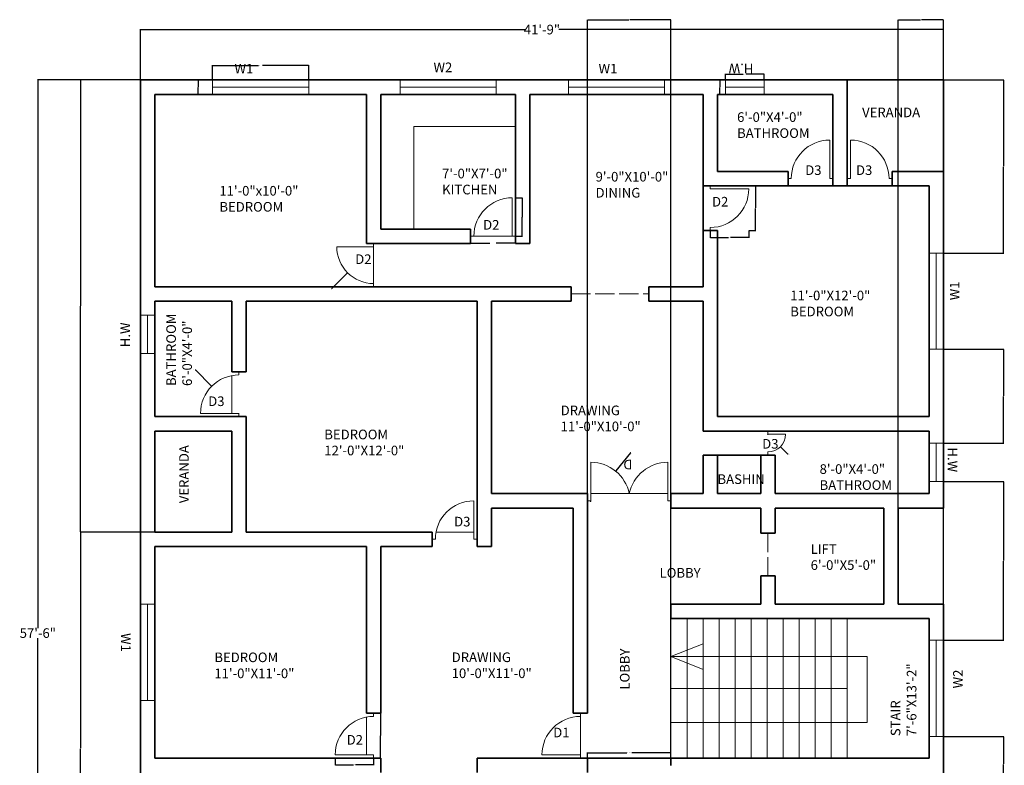
# Model space of a CAD drawing. Units: inches. Extents: x -51 to 563, y -718 to 47.
# Tile 2 of 2: x -51 to 563, y -418 to 47. Entities that reach past the tile are written whole.
import ezdxf

# ---------------------------------------------------------------- set-up
doc = ezdxf.new("R2010")
doc.units = ezdxf.units.IN
doc.header["$MEASUREMENT"] = 0
doc.linetypes.add('ACAD_ISO02W100', pattern=[15, 12, -3])
for name, color, linetype, lineweight in [('A-ANNO-DIMS', 2, 'Continuous', 18), ('A-ANNO-TEXT', 7, 'Continuous', 18), ('A-AREA-IDEN', 7, 'Continuous', 18), ('A-DOOR', 3, 'Continuous', 18), ('A-FLOR-CASE', 9, 'Continuous', 18), ('A-FLOR-STRS', 7, 'Continuous', 18), ('A-GLAZ', 164, 'Continuous', 18), ('A-WALL', 7, 'Continuous', 35), ('A-WALL-OPEN', 8, 'ACAD_ISO02W100', 13)]:
    doc.layers.add(name, color=color, linetype=linetype, lineweight=lineweight)
doc.styles.get("Standard").update_dxf_attribs({"font": 'arial.ttf'})
doc.dimstyles.get("Standard").update_dxf_attribs({"dimtxt": 0.18, "dimasz": 0.18, "dimexe": 0.18, "dimexo": 0.0625, "dimgap": 0.09, "dimtad": 0, "dimtih": 1, "dimtoh": 1, "dimdec": 0, "dimzin": 0, "dimdsep": 46, "dimlunit": 3, "dimtxsty": 'Standard', "dimcen": 0.09, "dimadec": 0, "dimazin": 0, "dimtfac": 1, "dimtdec": 0, "dimtofl": 0, "dimtmove": 0, "dimatfit": 3, "dimfxl": 1, "dimtolj": 1, "dimtzin": 0, "dimarcsym": 0})

# ---------------------------------------------------------------- blocks, each defined once
blk = doc.blocks.new('*D1')
at = {"layer": 'A-ANNO-DIMS', "color": 0, "lineweight": -2, "transparency": 16777216}
for p, q in [((24.24, 9.78), (24.24, 41.31)), ((24.42, 41.13), (264.22, 41.13)), ((525.06, 41.13), (285.25, 41.13)), ((525.24, 9.78), (525.24, 41.31))]:
    blk.add_line(p, q, dxfattribs=at)
at = {"layer": 'A-ANNO-DIMS', "color": 0, "transparency": 16777216}
for points in [[(24.42, 41.16), (24.42, 41.1), (24.24, 41.13)], [(525.06, 41.16), (525.06, 41.1), (525.24, 41.13)]]:
    blk.add_solid(points, dxfattribs=at)
at = {"layer": 'Defpoints', "color": 0, "transparency": 16777216}
for p in [(525.24, 41.13), (24.24, 9.71), (525.24, 9.71)]:
    blk.add_point(p, dxfattribs=at)
at = {"layer": 'A-ANNO-DIMS', "color": 0, "transparency": 16777216, "insert": (274.74, 41.13), "char_height": 6, "attachment_point": 5}
blk.add_mtext('\\A1;41\'-9"', dxfattribs=at)
blk = doc.blocks.new('*D2')
at = {"layer": 'A-ANNO-DIMS', "color": 0, "lineweight": -2, "transparency": 16777216}
for p, q in [((24.17, 9.71), (-39.93, 9.71)), ((-39.75, 9.53), (-39.75, -332.13)), ((-39.75, -680.11), (-39.75, -338.44)), ((24.17, -680.29), (-39.93, -680.29))]:
    blk.add_line(p, q, dxfattribs=at)
at = {"layer": 'A-ANNO-DIMS', "color": 0, "transparency": 16777216}
for points in [[(-39.78, 9.53), (-39.72, 9.53), (-39.75, 9.71)], [(-39.78, -680.11), (-39.72, -680.11), (-39.75, -680.29)]]:
    blk.add_solid(points, dxfattribs=at)
at = {"layer": 'Defpoints', "color": 0, "transparency": 16777216}
for p in [(24.24, 9.71), (-39.75, -680.29), (24.24, -680.29)]:
    blk.add_point(p, dxfattribs=at)
at = {"layer": 'A-ANNO-DIMS', "color": 0, "transparency": 16777216, "insert": (-39.75, -335.29), "char_height": 6, "attachment_point": 5}
blk.add_mtext('\\A1;57\'-6"', dxfattribs=at)
blk = doc.blocks.new('WIN-60IN')
for p, q in [((0, 9), (60, 9)), ((0, 0), (0, 9)), ((60, 9), (60, 0)), ((0, 4.5), (60, 4.5)), ((60, 0), (0, 0))]:
    blk.add_line(p, q)
blk = doc.blocks.new('WIN-24IN')
for p, q in [((0, 9), (24, 9)), ((0, 0), (0, 9)), ((24, 9), (24, 0)), ((0, 4.5), (24, 4.5)), ((24, 0), (0, 0))]:
    blk.add_line(p, q)
blk = doc.blocks.new('DOOR-24IN-CENTER-THRESHOLD')
for p, q in [((26, 0), (26, 24)), ((2, 0), (0, 0)), ((2, 0), (26, 0)), ((28, 0), (26, 0))]:
    blk.add_line(p, q)
blk.add_arc((26, 0), 24, 90, 180)
blk = doc.blocks.new('DOOR-24IN-SWING')
for p, q in [((26, 0), (26, 24)), ((2, 0), (0, 0)), ((28, 0), (26, 0))]:
    blk.add_line(p, q)
blk.add_arc((26, 0), 24, 90, 180)
blk = doc.blocks.new('DOOR-24IN-OFFSET-THRESHOLD')
for p, q in [((19.5, 25.57), (19.5, 2)), ((24, 26), (24, 28)), ((24, 2), (0, 2)), ((24, 0), (24, 2))]:
    blk.add_line(p, q)
blk.add_arc((24, 2), 24, 90, 180)
blk = doc.blocks.new('DOOR-48IN-PAIR')
for p, q in [((2, 0), (2, 24)), ((50, 0), (50, 24)), ((0, 0), (2, 0)), ((50, 0), (52, 0))]:
    blk.add_line(p, q)
for centre, start, end in [((2, -0.52), 11.81228, 90), ((50, -0.52), 90, 168.18772)]:
    blk.add_arc(centre, 24.52, start, end)
blk = doc.blocks.new('*D9')
at = {"layer": 'A-ANNO-DIMS', "color": 0, "lineweight": -2, "transparency": 16777216}
for p, q in [((69.24, 9.78), (69.24, 18.89)), ((69.42, 18.71), (98.01, 18.71)), ((129.06, 18.71), (100.47, 18.71)), ((129.24, 9.78), (129.24, 18.89))]:
    blk.add_line(p, q, dxfattribs=at)
at = {"layer": 'A-ANNO-DIMS', "color": 0, "transparency": 16777216}
for points in [[(69.42, 18.74), (69.42, 18.68), (69.24, 18.71)], [(129.06, 18.74), (129.06, 18.68), (129.24, 18.71)]]:
    blk.add_solid(points, dxfattribs=at)
at = {"layer": 'Defpoints', "color": 0, "transparency": 16777216}
for p in [(129.24, 18.71), (69.24, 9.71), (129.24, 9.71)]:
    blk.add_point(p, dxfattribs=at)
at = {"layer": 'A-ANNO-DIMS', "color": 0, "transparency": 16777216, "insert": (99.24, 18.71), "char_height": 0.18, "attachment_point": 5}
blk.add_mtext('\\A1;WINDOW 5\'-0" TYP.', dxfattribs=at)
blk = doc.blocks.new('*D10')
at = {"layer": 'A-ANNO-DIMS', "color": 0, "lineweight": -2, "transparency": 16777216}
for p, q in [((69.17, 9.71), (60.06, 9.71)), ((60.24, 9.53), (60.24, 5.4)), ((69.17, 0.71), (60.06, 0.71)), ((60.24, 0.89), (60.24, 5.03))]:
    blk.add_line(p, q, dxfattribs=at)
at = {"layer": 'A-ANNO-DIMS', "color": 0, "transparency": 16777216}
for points in [[(60.21, 9.53), (60.27, 9.53), (60.24, 9.71)], [(60.21, 0.89), (60.27, 0.89), (60.24, 0.71)]]:
    blk.add_solid(points, dxfattribs=at)
at = {"layer": 'Defpoints', "color": 0, "transparency": 16777216}
for p in [(60.24, 9.71), (69.24, 9.71), (69.24, 0.71)]:
    blk.add_point(p, dxfattribs=at)
at = {"layer": 'A-ANNO-DIMS', "color": 0, "transparency": 16777216, "insert": (60.24, 5.21), "char_height": 0.18, "attachment_point": 5}
blk.add_mtext('\\A1;0\'-9" TYP.', dxfattribs=at)
blk = doc.blocks.new('*D11')
at = {"layer": 'A-ANNO-DIMS', "color": 0, "lineweight": -2, "transparency": 16777216}
for p, q in [((389.26, 9.78), (389.26, 13.49)), ((389.44, 13.31), (400.31, 13.31)), ((413.08, 13.31), (402.21, 13.31)), ((413.26, 9.78), (413.26, 13.49))]:
    blk.add_line(p, q, dxfattribs=at)
at = {"layer": 'A-ANNO-DIMS', "color": 0, "transparency": 16777216}
for points in [[(389.44, 13.34), (389.44, 13.28), (389.26, 13.31)], [(413.08, 13.34), (413.08, 13.28), (413.26, 13.31)]]:
    blk.add_solid(points, dxfattribs=at)
at = {"layer": 'Defpoints', "color": 0, "transparency": 16777216}
for p in [(389.26, 13.31), (389.26, 9.71), (413.26, 9.71)]:
    blk.add_point(p, dxfattribs=at)
at = {"layer": 'A-ANNO-DIMS', "color": 0, "transparency": 16777216, "insert": (401.26, 13.31), "char_height": 0.18, "attachment_point": 5}
blk.add_mtext('\\A1;H.W. 2\'-0" TYP.', dxfattribs=at)
blk = doc.blocks.new('*D12')
at = {"layer": 'A-ANNO-DIMS', "color": 0, "lineweight": -2, "transparency": 16777216}
for p, q in [((389.2, 9.71), (385.48, 9.71)), ((385.66, 9.53), (385.66, 5.4)), ((389.2, 0.71), (385.48, 0.71)), ((385.66, 0.89), (385.66, 5.03))]:
    blk.add_line(p, q, dxfattribs=at)
at = {"layer": 'A-ANNO-DIMS', "color": 0, "transparency": 16777216}
for points in [[(385.63, 9.53), (385.69, 9.53), (385.66, 9.71)], [(385.63, 0.89), (385.69, 0.89), (385.66, 0.71)]]:
    blk.add_solid(points, dxfattribs=at)
at = {"layer": 'Defpoints', "color": 0, "transparency": 16777216}
for p in [(389.26, 9.71), (385.66, 0.71), (389.26, 0.71)]:
    blk.add_point(p, dxfattribs=at)
at = {"layer": 'A-ANNO-DIMS', "color": 0, "transparency": 16777216, "insert": (385.66, 5.21), "char_height": 0.18, "attachment_point": 5}
blk.add_mtext('\\A1;0\'-9" TYP.', dxfattribs=at)
blk = doc.blocks.new('*D13')
at = {"layer": 'A-ANNO-DIMS', "color": 0, "lineweight": -2, "transparency": 16777216}
for p, q in [((169.8, -385.29), (174.12, -385.29)), ((173.94, -385.47), (173.94, -399.1)), ((173.94, -413.11), (173.94, -399.47)), ((169.8, -413.29), (174.12, -413.29))]:
    blk.add_line(p, q, dxfattribs=at)
at = {"layer": 'A-ANNO-DIMS', "color": 0, "transparency": 16777216}
for points in [[(173.91, -385.47), (173.97, -385.47), (173.94, -385.29)], [(173.91, -413.11), (173.97, -413.11), (173.94, -413.29)]]:
    blk.add_solid(points, dxfattribs=at)
at = {"layer": 'Defpoints', "color": 0, "transparency": 16777216}
for p in [(169.74, -385.29), (173.94, -385.29), (169.74, -413.29)]:
    blk.add_point(p, dxfattribs=at)
at = {"layer": 'A-ANNO-DIMS', "color": 0, "transparency": 16777216, "insert": (173.94, -399.29), "char_height": 0.18, "attachment_point": 5}
blk.add_mtext('\\A1;OFFSET THRESHOLD 2\'-4" TYP.', dxfattribs=at)
blk = doc.blocks.new('*D14')
at = {"layer": 'A-ANNO-DIMS', "color": 0, "lineweight": -2, "transparency": 16777216}
for p, q in [((145.74, -413.35), (145.74, -417.67)), ((145.92, -417.49), (157.1, -417.49)), ((169.56, -417.49), (158.38, -417.49)), ((169.74, -413.35), (169.74, -417.67))]:
    blk.add_line(p, q, dxfattribs=at)
at = {"layer": 'A-ANNO-DIMS', "color": 0, "transparency": 16777216}
for points in [[(145.92, -417.46), (145.92, -417.52), (145.74, -417.49)], [(169.56, -417.46), (169.56, -417.52), (169.74, -417.49)]]:
    blk.add_solid(points, dxfattribs=at)
at = {"layer": 'Defpoints', "color": 0, "transparency": 16777216}
for p in [(145.74, -413.29), (169.74, -413.29), (169.74, -417.49)]:
    blk.add_point(p, dxfattribs=at)
at = {"layer": 'A-ANNO-DIMS', "color": 0, "transparency": 16777216, "insert": (157.74, -417.49), "char_height": 0.18, "attachment_point": 5}
blk.add_mtext('\\A1;2\'-0" TYP.', dxfattribs=at)
blk = doc.blocks.new('*D15')
at = {"layer": 'A-ANNO-DIMS', "color": 0, "lineweight": -2, "transparency": 16777216}
for p, q in [((403.8, -56.29), (408.12, -56.29)), ((407.94, -56.47), (407.94, -70.1)), ((407.94, -84.11), (407.94, -70.47)), ((403.8, -84.29), (408.12, -84.29))]:
    blk.add_line(p, q, dxfattribs=at)
at = {"layer": 'A-ANNO-DIMS', "color": 0, "transparency": 16777216}
for points in [[(407.91, -56.47), (407.97, -56.47), (407.94, -56.29)], [(407.91, -84.11), (407.97, -84.11), (407.94, -84.29)]]:
    blk.add_solid(points, dxfattribs=at)
at = {"layer": 'Defpoints', "color": 0, "transparency": 16777216}
for p in [(403.74, -56.29), (407.94, -56.29), (403.74, -84.29)]:
    blk.add_point(p, dxfattribs=at)
at = {"layer": 'A-ANNO-DIMS', "color": 0, "transparency": 16777216, "insert": (407.94, -70.29), "char_height": 0.18, "attachment_point": 5}
blk.add_mtext('\\A1;SWING DOOR 2\'-4" TYP.', dxfattribs=at)
blk = doc.blocks.new('*D16')
at = {"layer": 'A-ANNO-DIMS', "color": 0, "lineweight": -2, "transparency": 16777216}
for p, q in [((379.74, -84.35), (379.74, -88.67)), ((403.74, -84.35), (403.74, -88.67)), ((379.92, -88.49), (391.1, -88.49)), ((403.56, -88.49), (392.38, -88.49))]:
    blk.add_line(p, q, dxfattribs=at)
at = {"layer": 'A-ANNO-DIMS', "color": 0, "transparency": 16777216}
for points in [[(379.92, -88.46), (379.92, -88.52), (379.74, -88.49)], [(403.56, -88.46), (403.56, -88.52), (403.74, -88.49)]]:
    blk.add_solid(points, dxfattribs=at)
at = {"layer": 'Defpoints', "color": 0, "transparency": 16777216}
for p in [(379.74, -84.29), (403.74, -84.29), (403.74, -88.49)]:
    blk.add_point(p, dxfattribs=at)
at = {"layer": 'A-ANNO-DIMS', "color": 0, "transparency": 16777216, "insert": (391.74, -88.49), "char_height": 0.18, "attachment_point": 5}
blk.add_mtext('\\A1;2\'-0" TYP.', dxfattribs=at)
blk = doc.blocks.new('*D17')
at = {"layer": 'A-ANNO-DIMS', "color": 0, "lineweight": -2, "transparency": 16777216}
for p, q in [((230.24, -87.85), (230.24, -92.17)), ((230.42, -91.99), (242.24, -91.99)), ((258.06, -91.99), (246.24, -91.99)), ((258.24, -87.85), (258.24, -92.17))]:
    blk.add_line(p, q, dxfattribs=at)
at = {"layer": 'A-ANNO-DIMS', "color": 0, "transparency": 16777216}
for points in [[(230.42, -91.96), (230.42, -92.02), (230.24, -91.99)], [(258.06, -91.96), (258.06, -92.02), (258.24, -91.99)]]:
    blk.add_solid(points, dxfattribs=at)
at = {"layer": 'Defpoints', "color": 0, "transparency": 16777216}
for p in [(230.24, -87.79), (258.24, -87.79), (258.24, -91.99)]:
    blk.add_point(p, dxfattribs=at)
at = {"layer": 'A-ANNO-DIMS', "color": 0, "transparency": 16777216, "insert": (244.24, -91.99), "char_height": 0.18, "attachment_point": 5}
blk.add_mtext('\\A1;CENTER THRESHOLD 2\'-4" TYP.', dxfattribs=at)
blk = doc.blocks.new('*D18')
at = {"layer": 'A-ANNO-DIMS', "color": 0, "lineweight": -2, "transparency": 16777216}
for p, q in [((258.3, -63.79), (262.62, -63.79)), ((262.44, -63.97), (262.44, -75.6)), ((262.44, -87.61), (262.44, -75.97)), ((258.3, -87.79), (262.62, -87.79))]:
    blk.add_line(p, q, dxfattribs=at)
at = {"layer": 'A-ANNO-DIMS', "color": 0, "transparency": 16777216}
for points in [[(262.41, -63.97), (262.47, -63.97), (262.44, -63.79)], [(262.41, -87.61), (262.47, -87.61), (262.44, -87.79)]]:
    blk.add_solid(points, dxfattribs=at)
at = {"layer": 'Defpoints', "color": 0, "transparency": 16777216}
for p in [(258.24, -63.79), (262.44, -63.79), (258.24, -87.79)]:
    blk.add_point(p, dxfattribs=at)
at = {"layer": 'A-ANNO-DIMS', "color": 0, "transparency": 16777216, "insert": (262.44, -75.79), "char_height": 0.18, "attachment_point": 5}
blk.add_mtext('\\A1;2\'-0" TYP.', dxfattribs=at)
blk = doc.blocks.new('*D19')
at = {"layer": 'A-ANNO-DIMS', "color": 0, "lineweight": -2, "transparency": 16777216}
for p, q in [((303.24, -417.72), (303.24, -409.81)), ((303.42, -409.99), (327.69, -409.99)), ((355.06, -409.99), (330.79, -409.99)), ((355.24, -417.72), (355.24, -409.81))]:
    blk.add_line(p, q, dxfattribs=at)
at = {"layer": 'A-ANNO-DIMS', "color": 0, "transparency": 16777216}
for points in [[(303.42, -409.96), (303.42, -410.02), (303.24, -409.99)], [(355.06, -409.96), (355.06, -410.02), (355.24, -409.99)]]:
    blk.add_solid(points, dxfattribs=at)
at = {"layer": 'Defpoints', "color": 0, "transparency": 16777216}
for p in [(303.24, -409.99), (303.24, -417.79), (355.24, -417.79)]:
    blk.add_point(p, dxfattribs=at)
at = {"layer": 'A-ANNO-DIMS', "color": 0, "transparency": 16777216, "insert": (329.24, -409.99), "char_height": 0.18, "attachment_point": 5}
blk.add_mtext('\\A1;PAIRED DOOR 4\'-4" TYP.', dxfattribs=at)
blk = doc.blocks.new('*D25')
at = {"layer": 'A-ANNO-DIMS', "color": 0, "lineweight": -2, "transparency": 16777216}
for p, q in [((24.17, 9.71), (-13.34, 9.71)), ((-13.16, 9.53), (-13.16, -131.1)), ((-13.16, -272.11), (-13.16, -131.47)), ((33.17, -272.29), (-13.34, -272.29))]:
    blk.add_line(p, q, dxfattribs=at)
at = {"layer": 'A-ANNO-DIMS', "color": 0, "transparency": 16777216}
for points in [[(-13.19, 9.53), (-13.13, 9.53), (-13.16, 9.71)], [(-13.19, -272.11), (-13.13, -272.11), (-13.16, -272.29)]]:
    blk.add_solid(points, dxfattribs=at)
at = {"layer": 'Defpoints', "color": 0, "transparency": 16777216}
for p in [(24.24, 9.71), (-13.16, -272.29), (33.24, -272.29)]:
    blk.add_point(p, dxfattribs=at)
at = {"layer": 'A-ANNO-DIMS', "color": 0, "transparency": 16777216, "insert": (-13.16, -131.29), "char_height": 0.18, "attachment_point": 5}
blk.add_mtext('\\A1;23\'-6"', dxfattribs=at)
blk = doc.blocks.new('*D26')
at = {"layer": 'A-ANNO-DIMS', "color": 0, "lineweight": -2, "transparency": 16777216}
for p, q in [((33.17, -272.29), (-13.34, -272.29)), ((-13.16, -272.47), (-13.16, -407.1)), ((-13.16, -542.11), (-13.16, -407.47)), ((33.17, -542.29), (-13.34, -542.29))]:
    blk.add_line(p, q, dxfattribs=at)
at = {"layer": 'A-ANNO-DIMS', "color": 0, "transparency": 16777216}
for points in [[(-13.19, -272.47), (-13.13, -272.47), (-13.16, -272.29)], [(-13.19, -542.11), (-13.13, -542.11), (-13.16, -542.29)]]:
    blk.add_solid(points, dxfattribs=at)
at = {"layer": 'Defpoints', "color": 0, "transparency": 16777216}
for p in [(33.24, -272.29), (-13.16, -542.29), (33.24, -542.29)]:
    blk.add_point(p, dxfattribs=at)
at = {"layer": 'A-ANNO-DIMS', "color": 0, "transparency": 16777216, "insert": (-13.16, -407.29), "char_height": 0.18, "attachment_point": 5}
blk.add_mtext('\\A1;22\'-6"', dxfattribs=at)
blk = doc.blocks.new('*D28')
at = {"layer": 'A-ANNO-DIMS', "color": 0, "lineweight": -2, "transparency": 16777216}
for p, q in [((525.3, 9.71), (562.82, 9.71)), ((562.64, 9.53), (562.64, -44.1)), ((562.64, -98.11), (562.64, -44.47)), ((525.3, -98.29), (562.82, -98.29))]:
    blk.add_line(p, q, dxfattribs=at)
at = {"layer": 'A-ANNO-DIMS', "color": 0, "transparency": 16777216}
for points in [[(562.61, 9.53), (562.67, 9.53), (562.64, 9.71)], [(562.61, -98.11), (562.67, -98.11), (562.64, -98.29)]]:
    blk.add_solid(points, dxfattribs=at)
at = {"layer": 'Defpoints', "color": 0, "transparency": 16777216}
for p in [(525.24, 9.71), (525.24, -98.29), (562.64, -98.29)]:
    blk.add_point(p, dxfattribs=at)
at = {"layer": 'A-ANNO-DIMS', "color": 0, "transparency": 16777216, "insert": (562.64, -44.29), "char_height": 0.18, "attachment_point": 5}
blk.add_mtext('\\A1;9\'-0"', dxfattribs=at)
blk = doc.blocks.new('*D29')
at = {"layer": 'A-ANNO-DIMS', "color": 0, "lineweight": -2, "transparency": 16777216}
for p, q in [((525.3, -158.29), (562.82, -158.29)), ((562.64, -158.47), (562.64, -187.35)), ((562.64, -216.61), (562.64, -187.72)), ((525.3, -216.79), (562.82, -216.79))]:
    blk.add_line(p, q, dxfattribs=at)
at = {"layer": 'A-ANNO-DIMS', "color": 0, "transparency": 16777216}
for points in [[(562.61, -158.47), (562.67, -158.47), (562.64, -158.29)], [(562.61, -216.61), (562.67, -216.61), (562.64, -216.79)]]:
    blk.add_solid(points, dxfattribs=at)
at = {"layer": 'Defpoints', "color": 0, "transparency": 16777216}
for p in [(525.24, -158.29), (525.24, -216.79), (562.64, -216.79)]:
    blk.add_point(p, dxfattribs=at)
at = {"layer": 'A-ANNO-DIMS', "color": 0, "transparency": 16777216, "insert": (562.64, -187.54), "char_height": 0.18, "attachment_point": 5}
blk.add_mtext('\\A1;4\'-10 1/2"', dxfattribs=at)
blk = doc.blocks.new('*D30')
at = {"layer": 'A-ANNO-DIMS', "color": 0, "lineweight": -2, "transparency": 16777216}
for p, q in [((525.3, -240.79), (562.82, -240.79)), ((562.64, -240.97), (562.64, -290.1)), ((562.64, -339.61), (562.64, -290.47)), ((525.3, -339.79), (562.82, -339.79))]:
    blk.add_line(p, q, dxfattribs=at)
at = {"layer": 'A-ANNO-DIMS', "color": 0, "transparency": 16777216}
for points in [[(562.61, -240.97), (562.67, -240.97), (562.64, -240.79)], [(562.61, -339.61), (562.67, -339.61), (562.64, -339.79)]]:
    blk.add_solid(points, dxfattribs=at)
at = {"layer": 'Defpoints', "color": 0, "transparency": 16777216}
for p in [(525.24, -240.79), (525.24, -339.79), (562.64, -339.79)]:
    blk.add_point(p, dxfattribs=at)
at = {"layer": 'A-ANNO-DIMS', "color": 0, "transparency": 16777216, "insert": (562.64, -290.29), "char_height": 0.18, "attachment_point": 5}
blk.add_mtext('\\A1;8\'-3"', dxfattribs=at)
blk = doc.blocks.new('*D31')
at = {"layer": 'A-ANNO-DIMS', "color": 0, "lineweight": -2, "transparency": 16777216}
for p, q in [((525.3, -399.79), (562.82, -399.79)), ((562.64, -399.97), (562.64, -416.85)), ((562.64, -434.11), (562.64, -417.22)), ((525.3, -434.29), (562.82, -434.29))]:
    blk.add_line(p, q, dxfattribs=at)
at = {"layer": 'A-ANNO-DIMS', "color": 0, "transparency": 16777216}
for points in [[(562.61, -399.97), (562.67, -399.97), (562.64, -399.79)], [(562.61, -434.11), (562.67, -434.11), (562.64, -434.29)]]:
    blk.add_solid(points, dxfattribs=at)
at = {"layer": 'Defpoints', "color": 0, "transparency": 16777216}
for p in [(525.24, -399.79), (525.24, -434.29), (562.64, -434.29)]:
    blk.add_point(p, dxfattribs=at)
at = {"layer": 'A-ANNO-DIMS', "color": 0, "transparency": 16777216, "insert": (562.64, -417.04), "char_height": 0.18, "attachment_point": 5}
blk.add_mtext('\\A1;2\'-10 1/2"', dxfattribs=at)
blk = doc.blocks.new('*D33')
at = {"layer": 'A-ANNO-DIMS', "color": 0, "lineweight": -2, "transparency": 16777216}
for p, q in [((497.04, -317.22), (497.04, 47.29)), ((497.22, 47.11), (510.81, 47.11)), ((525.06, 47.11), (511.47, 47.11)), ((525.24, -317.22), (525.24, 47.29))]:
    blk.add_line(p, q, dxfattribs=at)
at = {"layer": 'A-ANNO-DIMS', "color": 0, "transparency": 16777216}
for points in [[(497.22, 47.14), (497.22, 47.08), (497.04, 47.11)], [(525.06, 47.14), (525.06, 47.08), (525.24, 47.11)]]:
    blk.add_solid(points, dxfattribs=at)
at = {"layer": 'Defpoints', "color": 0, "transparency": 16777216}
for p in [(525.24, 47.11), (497.04, -317.29), (525.24, -317.29)]:
    blk.add_point(p, dxfattribs=at)
at = {"layer": 'A-ANNO-DIMS', "color": 0, "transparency": 16777216, "insert": (511.14, 47.11), "char_height": 0.18, "attachment_point": 5}
blk.add_mtext('\\A1;2\'-4"', dxfattribs=at)
blk = doc.blocks.new('*D34')
at = {"layer": 'A-ANNO-DIMS', "color": 0, "lineweight": -2, "transparency": 16777216}
for p, q in [((303.24, -385.22), (303.24, 47.29)), ((303.42, 47.11), (328.9, 47.11)), ((355.06, 47.11), (329.57, 47.11)), ((355.24, -413.22), (355.24, 47.29))]:
    blk.add_line(p, q, dxfattribs=at)
at = {"layer": 'A-ANNO-DIMS', "color": 0, "transparency": 16777216}
for points in [[(303.42, 47.14), (303.42, 47.08), (303.24, 47.11)], [(355.06, 47.14), (355.06, 47.08), (355.24, 47.11)]]:
    blk.add_solid(points, dxfattribs=at)
at = {"layer": 'Defpoints', "color": 0, "transparency": 16777216}
for p in [(355.24, 47.11), (303.24, -385.29), (355.24, -413.29)]:
    blk.add_point(p, dxfattribs=at)
at = {"layer": 'A-ANNO-DIMS', "color": 0, "transparency": 16777216, "insert": (329.24, 47.11), "char_height": 0.18, "attachment_point": 5}
blk.add_mtext('\\A1;4\'-4"', dxfattribs=at)
blk = doc.blocks.new('*D35')
at = {"layer": 'A-ANNO-DIMS', "color": 0, "lineweight": -2, "transparency": 16777216}
for p, q in [((329.97, -222.86), (320.81, -234.14)), ((330.15, -222.86), (329.97, -222.86)), ((305.15, -253.31), (305.33, -253.31)), ((305.24, -253.4), (305.24, -253.22))]:
    blk.add_line(p, q, dxfattribs=at)
at = {"layer": 'A-ANNO-DIMS', "color": 0, "transparency": 16777216}
blk.add_solid([(320.79, -234.12), (320.83, -234.15), (320.7, -234.28)], dxfattribs=at)
at = {"layer": 'Defpoints', "color": 0, "transparency": 16777216}
for p in [(320.7, -234.28), (305.24, -253.31)]:
    blk.add_point(p, dxfattribs=at)
at = {"layer": 'A-ANNO-DIMS', "color": 0, "transparency": 16777216, "insert": (330.98, -222.86), "char_height": 0.18, "attachment_point": 5}
blk.add_mtext('\\A1;4X R2\'-0 1/2"', dxfattribs=at)
blk = doc.blocks.new('*D36')
at = {"layer": 'A-ANNO-DIMS', "color": 0, "lineweight": -2, "transparency": 16777216}
for p, q in [((58.4, -171.13), (58.58, -171.13)), ((58.58, -171.13), (68.64, -181.19)), ((85.65, -198.29), (85.83, -198.29)), ((85.74, -198.38), (85.74, -198.2))]:
    blk.add_line(p, q, dxfattribs=at)
at = {"layer": 'A-ANNO-DIMS', "color": 0, "transparency": 16777216}
blk.add_solid([(68.66, -181.17), (68.62, -181.21), (68.77, -181.32)], dxfattribs=at)
at = {"layer": 'Defpoints', "color": 0, "transparency": 16777216}
for p in [(68.77, -181.32), (85.74, -198.29)]:
    blk.add_point(p, dxfattribs=at)
at = {"layer": 'A-ANNO-DIMS', "color": 0, "transparency": 16777216, "insert": (57.8, -171.13), "char_height": 0.18, "attachment_point": 5}
blk.add_mtext('\\A1;7X R2\'-0"', dxfattribs=at)
blk = doc.blocks.new('*D38')
at = {"layer": 'A-ANNO-DIMS', "color": 0, "lineweight": -2, "transparency": 16777216}
for p, q in [((169.65, -94.29), (169.83, -94.29)), ((169.74, -94.38), (169.74, -94.2)), ((143.71, -120.31), (153.35, -110.68)), ((143.53, -120.31), (143.71, -120.31))]:
    blk.add_line(p, q, dxfattribs=at)
at = {"layer": 'A-ANNO-DIMS', "color": 0, "transparency": 16777216}
blk.add_solid([(153.32, -110.66), (153.37, -110.7), (153.47, -110.55)], dxfattribs=at)
at = {"layer": 'Defpoints', "color": 0, "transparency": 16777216}
for p in [(169.74, -94.29), (153.47, -110.55)]:
    blk.add_point(p, dxfattribs=at)
at = {"layer": 'A-ANNO-DIMS', "color": 0, "transparency": 16777216, "insert": (143.05, -120.31), "char_height": 0.18, "attachment_point": 5}
blk.add_mtext('\\A1;R1\'-11"', dxfattribs=at)
blk = doc.blocks.new('*D40')
at = {"layer": 'A-ANNO-DIMS', "color": 0, "lineweight": -2, "transparency": 16777216}
for p, q in [((415.65, -211.29), (415.83, -211.29)), ((415.74, -211.38), (415.74, -211.2)), ((428.18, -223.73), (423.64, -219.19)), ((428.36, -223.73), (428.18, -223.73))]:
    blk.add_line(p, q, dxfattribs=at)
at = {"layer": 'A-ANNO-DIMS', "color": 0, "transparency": 16777216}
blk.add_solid([(423.66, -219.17), (423.62, -219.21), (423.51, -219.06)], dxfattribs=at)
at = {"layer": 'Defpoints', "color": 0, "transparency": 16777216}
for p in [(415.74, -211.29), (423.51, -219.06)]:
    blk.add_point(p, dxfattribs=at)
at = {"layer": 'A-ANNO-DIMS', "color": 0, "transparency": 16777216, "insert": (428.85, -223.73), "char_height": 0.18, "attachment_point": 5}
blk.add_mtext('\\A1;R0\'-11"', dxfattribs=at)

msp = doc.modelspace()

# ---------------------------------------------------------------- linework, layer by layer
at = {"layer": 'A-DOOR'}
for p, q in [((169.74, -94.29), (146.74, -94.29)), ((169.74, -92.29), (169.74, -94.29)), ((169.74, -94.29), (169.74, -117.29)), ((169.74, -119.29), (169.74, -117.29)), ((415.74, -209.29), (415.74, -211.29)), ((415.74, -211.29), (426.74, -211.29)), ((415.74, -224.29), (415.74, -222.29)), ((305.24, -248.29), (353.24, -248.29))]:
    msp.add_line(p, q, dxfattribs=at)
for centre, radius, start, end in [((169.74, -94.29), 23, 180, 270), ((415.74, -211.29), 11, 270, 0)]:
    msp.add_arc(centre, radius, start, end, dxfattribs=at)
at = {"layer": 'A-FLOR-CASE'}
for p, q in [((258.24, -19.3), (194.72, -19.3)), ((194.72, -19.3), (194.72, -83.29))]:
    msp.add_line(p, q, dxfattribs=at)
at = {"layer": 'A-FLOR-STRS'}
for p, q in [((355.24, -326.29), (355.24, -413.29)), ((365.24, -326.29), (365.24, -413.29)), ((375.24, -326.29), (375.24, -413.29)), ((385.24, -326.29), (385.24, -413.29)), ((395.24, -326.29), (395.24, -413.29)), ((405.24, -326.29), (405.24, -413.29)), ((415.24, -326.29), (415.24, -413.29)), ((425.24, -326.29), (425.24, -413.29)), ((435.24, -326.29), (435.24, -413.29)), ((445.24, -326.29), (445.24, -413.29)), ((455.24, -326.29), (455.24, -413.29)), ((465.24, -326.29), (465.24, -413.29)), ((355.24, -349.99), (375.24, -341.96)), ((477.63, -349.99), (355.24, -349.99)), ((355.24, -349.99), (375.24, -358.03)), ((477.63, -391.11), (477.63, -349.99)), ((465.24, -369.79), (355.24, -369.79)), ((355.24, -391.11), (477.63, -391.11))]:
    msp.add_line(p, q, dxfattribs=at)
at = {"layer": 'A-WALL'}
for p, q in [((24.24, 9.71), (24.24, -680.29)), ((24.24, 9.71), (525.24, 9.71)), ((465.24, 9.71), (465.24, -47.29)), ((525.24, 9.71), (525.24, -119.29)), ((33.24, 0.71), (165.24, 0.71)), ((33.24, 0.71), (33.24, -119.29)), ((165.24, 0.71), (165.24, -92.29)), ((174.24, 0.71), (174.24, -83.29)), ((174.24, 0.71), (258.24, 0.71)), ((258.24, 0.71), (258.24, -83.29)), ((267.24, 0.71), (267.24, -92.29)), ((267.24, 0.71), (375.24, 0.71)), ((375.24, 0.71), (375.24, -119.29)), ((384.24, 0.71), (384.24, -47.29)), ((384.24, 0.71), (456.24, 0.71)), ((456.24, 0.71), (456.24, -47.29)), ((384.24, -47.29), (428.24, -47.29)), ((428.24, -51.79), (428.24, -47.29)), ((456.24, -47.29), (456.24, -56.29)), ((465.24, -47.29), (465.24, -56.29)), ((493.24, -47.29), (525.24, -47.29)), ((493.24, -51.79), (493.24, -47.29)), ((428.24, -51.79), (428.24, -56.29)), ((493.24, -51.79), (493.24, -56.29)), ((384.24, -56.29), (375.24, -56.29)), ((384.24, -56.29), (516.24, -56.29)), ((516.24, -56.29), (516.24, -119.29)), ((516.24, -56.29), (516.24, -200.29)), ((525.24, -56.29), (525.24, -257.29)), ((174.24, -83.29), (230.24, -83.29)), ((230.24, -87.79), (230.24, -83.29)), ((258.24, -83.29), (258.24, -92.29)), ((379.74, -84.29), (375.24, -84.29)), ((379.74, -84.29), (384.24, -84.29)), ((384.24, -84.29), (384.24, -128.29)), ((230.24, -87.79), (230.24, -92.29)), ((165.24, -92.29), (230.24, -92.29)), ((258.24, -92.29), (267.24, -92.29)), ((33.24, -119.29), (292.92, -119.29)), ((292.92, -119.29), (292.92, -128.29)), ((341.33, -119.29), (341.33, -128.29)), ((341.33, -119.29), (375.24, -119.29)), ((33.24, -128.29), (81.24, -128.29)), ((33.24, -128.29), (33.24, -200.29)), ((81.24, -128.29), (81.24, -172.29)), ((90.24, -128.29), (90.24, -172.29)), ((90.24, -128.29), (234.24, -128.29)), ((234.24, -128.29), (234.24, -272.29)), ((243.24, -128.29), (243.24, -248.29)), ((243.24, -128.29), (292.92, -128.29)), ((341.33, -128.29), (375.24, -128.29)), ((375.24, -128.29), (375.24, -209.29)), ((384.24, -128.29), (384.24, -200.29)), ((85.74, -172.29), (81.24, -172.29)), ((85.74, -172.29), (90.24, -172.29)), ((33.24, -200.29), (81.24, -200.29)), ((81.24, -200.29), (90.24, -200.29)), ((90.24, -200.29), (90.24, -272.29)), ((384.24, -200.29), (516.24, -200.29)), ((33.24, -209.29), (81.24, -209.29)), ((33.24, -209.29), (33.24, -272.29)), ((81.24, -209.29), (81.24, -272.29)), ((375.24, -209.29), (516.24, -209.29)), ((516.24, -209.29), (516.24, -248.29)), ((420.24, -224.29), (375.24, -224.29)), ((375.24, -224.29), (375.24, -248.29)), ((384.24, -224.29), (384.24, -248.29)), ((411.24, -224.29), (411.24, -248.29)), ((420.24, -224.29), (420.24, -248.29)), ((243.24, -248.29), (303.24, -248.29)), ((303.24, -257.29), (303.24, -248.29)), ((355.24, -252.79), (355.24, -248.29)), ((355.24, -248.29), (375.24, -248.29)), ((384.24, -248.29), (411.24, -248.29)), ((420.24, -248.29), (516.24, -248.29)), ((243.24, -257.29), (294.24, -257.29)), ((243.24, -257.29), (243.24, -281.29)), ((294.24, -257.29), (294.24, -385.29)), ((303.24, -257.29), (303.24, -385.29)), ((355.24, -252.79), (355.24, -257.29)), ((355.24, -257.29), (411.24, -257.29)), ((411.24, -257.29), (411.24, -272.91)), ((420.24, -257.29), (420.24, -272.91)), ((420.24, -257.29), (488.04, -257.29)), ((488.04, -257.29), (488.04, -317.29)), ((497.04, -257.29), (497.04, -317.29)), ((497.04, -257.29), (525.24, -257.29)), ((33.24, -272.29), (81.24, -272.29)), ((90.24, -272.29), (206.24, -272.29)), ((206.24, -276.79), (206.24, -272.29)), ((234.24, -272.29), (234.24, -281.29)), ((420.24, -272.91), (411.24, -272.91)), ((33.24, -281.29), (165.24, -281.29)), ((33.24, -281.29), (33.24, -413.29)), ((165.24, -281.29), (165.24, -385.29)), ((174.24, -281.29), (174.24, -385.29)), ((174.24, -281.29), (206.24, -281.29)), ((206.24, -276.79), (206.24, -281.29)), ((234.24, -281.29), (243.24, -281.29)), ((411.24, -299.54), (420.24, -299.54)), ((411.24, -299.54), (411.24, -317.29)), ((420.24, -299.54), (420.24, -317.29)), ((355.24, -317.29), (411.24, -317.29)), ((355.24, -317.29), (355.24, -326.29)), ((420.24, -317.29), (488.04, -317.29)), ((497.04, -317.29), (525.24, -317.29)), ((525.24, -317.29), (525.24, -680.29)), ((355.24, -326.29), (516.24, -326.29)), ((516.24, -326.29), (516.24, -413.29)), ((169.74, -385.29), (165.24, -385.29)), ((169.74, -385.29), (174.24, -385.29)), ((298.74, -385.29), (294.24, -385.29)), ((298.74, -385.29), (303.24, -385.29)), ((33.24, -413.29), (165.24, -413.29)), ((165.24, -413.29), (174.24, -413.29)), ((174.24, -413.29), (174.24, -422.29)), ((234.24, -413.29), (294.24, -413.29)), ((234.24, -422.29), (234.24, -413.29)), ((294.24, -413.29), (303.24, -413.29)), ((303.24, -413.29), (516.24, -413.29)), ((303.24, -413.29), (303.24, -422.29)), ((355.24, -417.79), (355.24, -413.29))]:
    msp.add_line(p, q, dxfattribs=at)
at = {"layer": 'A-WALL-OPEN'}
for p, q in [((292.92, -123.79), (341.33, -123.79)), ((415.74, -272.91), (415.74, -299.54))]:
    msp.add_line(p, q, dxfattribs=at)

# ---------------------------------------------------------------- block references
at = {"layer": 'A-DOOR'}
for name, p in [('DOOR-24IN-SWING', (428.24, -51.79)), ('DOOR-24IN-CENTER-THRESHOLD', (230.24, -87.79)), ('DOOR-24IN-OFFSET-THRESHOLD', (61.74, -200.29)), ('DOOR-48IN-PAIR', (303.24, -252.79)), ('DOOR-24IN-OFFSET-THRESHOLD', (145.74, -413.29))]:
    msp.add_blockref(name, p, dxfattribs=at)
at = {"layer": 'A-DOOR', "extrusion": (0, 0, -1), "zscale": -1}
msp.add_blockref('DOOR-24IN-SWING', (-493.24, -51.79), dxfattribs=at)
for name, p, rotation in [('DOOR-24IN-SWING', (-379.74, -84.29), 90.00000000000006), ('DOOR-24IN-OFFSET-THRESHOLD', (-234.24, -252.79), 269.9999999999998), ('DOOR-24IN-CENTER-THRESHOLD', (-298.74, -385.29), 270)]:
    msp.add_blockref(name, p, dxfattribs=dict(at, rotation=rotation))
at = {"layer": 'A-GLAZ'}
for p in [(69.24, 0.71), (186.24, 0.71), (291.24, 0.71)]:
    msp.add_blockref('WIN-60IN', p, dxfattribs=at)
for name, p, rotation in [('WIN-24IN', (413.26, 9.71), 180), ('WIN-60IN', (525.24, -158.29), 90.00000000000003), ('WIN-24IN', (24.24, -137), 269.9999999999995), ('WIN-24IN', (516.24, -216.79), 269.9999999999996), ('WIN-60IN', (33.24, -377.29), 89.99999999999996), ('WIN-60IN', (525.24, -399.79), 89.99999999999996)]:
    msp.add_blockref(name, p, dxfattribs=dict(at, rotation=rotation))

# ---------------------------------------------------------------- texts
at = {"layer": 'A-ANNO-TEXT', "char_height": 6, "attachment_point": 1}
for s, insert in [('W1', (82.94, 19.76)), ('W2', (207.08, 20.56)), ('W1', (310.05, 19.76)), ('D3', (438.97, -43.55)), ('D3', (470.65, -43.55)), ('D2', (380.82, -63.23)), ('D2', (238.06, -77.65)), ('D2', (158.24, -99.08)), ('D3', (66.55, -187.68)), ('D3', (412.12, -214.24)), ('D3', (219.96, -262.77)), ('D2', (152.92, -398.87)), ('D1', (281.77, -394.32))]:
    msp.add_mtext(s, dxfattribs=dict(at, insert=insert))
for s, insert, rotation in [('H.W', (406.64, 13.84), 180), ('W1', (529.19, -127.7), 90), ('H.W', (11.8, -156.98), 90), ('H.W', (533.93, -219.52), 270), ('D', (331.15, -233.2), 180), ('W1', (18.21, -335.29), 270), ('W2', (531.26, -369.79), 90)]:
    msp.add_mtext(s, dxfattribs=dict(at, insert=insert, rotation=rotation))
at = {"layer": 'A-AREA-IDEN', "char_height": 6, "attachment_point": 1}
for s, insert in [('6\'-0"X4\'-0"\\PBATHROOM', (396.47, -10.45)), ('VERANDA', (474.45, -7.54)), ('7\'-0"X7\'-0"\\PKITCHEN', (212.43, -45.66)), ('11\'-0"x10\'-0"\\PBEDROOM', (73.51, -56.42)), ('11\'-0"X12\'-0"\\PBEDROOM', (429.64, -121.72)), ('DRAWING\\P11\'-0"X10\'-0"', (286.41, -193.39)), ('BEDROOM\\P12\'-0"X12\'-0"', (138.96, -208.41)), ('8\'-0"X4\'-0"\\PBATHROOM', (447.94, -229.99)), ('BASHIN', (384.24, -236.29)), ('LIFT\\P6\'-0"X5\'-0"', (442.35, -279.87)), ('LOBBY', (348.12, -294.71)), ('BEDROOM\\P11\'-0"X11\'-0"', (70.38, -347.42)), ('DRAWING\\P10\'-0"X11\'-0"', (218.43, -347.37))]:
    msp.add_mtext(s, dxfattribs=dict(at, insert=insert))
at = {"layer": 'A-AREA-IDEN', "insert": (308.19, -47.65), "char_height": 6, "width": 1.4297, "attachment_point": 1}
msp.add_mtext('9\'-0"X10\'-0"\\PDINING', dxfattribs=at)
at = {"layer": 'A-AREA-IDEN', "char_height": 6, "attachment_point": 1, "rotation": 90}
for s, insert in [('BATHROOM\\P6\'-0"X4\'-0"', (40.4, -181.19)), ('VERANDA', (48.43, -254.3)), ('STAIR\\P7\'-6"X13\'-2"', (492.34, -399.6))]:
    msp.add_mtext(s, dxfattribs=dict(at, insert=insert))
at = {"layer": 'A-AREA-IDEN', "insert": (323.39, -370.58), "char_height": 6, "attachment_point": 1, "rotation": 90}
msp.add_mtext_dynamic_manual_height_columns('LOBBY', width=2.2613, gutter_width=1, heights=[0], dxfattribs=at)

# ---------------------------------------------------------------- dimensions: what is measured, and where the dimension line sits
at = {"layer": 'A-ANNO-DIMS'}
for base, p1, p2, override, picture, middle in [((525.24, 41.13), (24.24, 9.71), (525.24, 9.71), {"dimtxt": 6, "dimclrd": 0, "dimclre": 0, "dimclrt": 0}, '*D1', (274.74, 41.13)), ((355.24, 47.11), (303.24, -385.29), (355.24, -413.29), {"dimdec": 1, "dimlfac": 1, "dimrnd": 0, "dimzin": 1, "dimdsep": 46, "dimlunit": 4, "dimfrac": 2}, '*D34', (329.24, 47.11)), ((525.24, 47.11), (497.04, -317.29), (525.24, -317.29), {"dimdec": 1, "dimlfac": 1, "dimrnd": 0, "dimzin": 1, "dimdsep": 46, "dimlunit": 4, "dimfrac": 2}, '*D33', (511.14, 47.11))]:
    dim = msp.add_linear_dim(base=base, p1=p1, p2=p2, dimstyle='Standard', override=override, dxfattribs=at)
    dim.commit()
    dim.dimension.update_dxf_attribs({"geometry": picture, "text_midpoint": middle})
for base, p1, p2, text, picture, middle in [((129.24, 18.71), (69.24, 9.71), (129.24, 9.71), 'WINDOW <> TYP.', '*D9', (99.24, 18.71)), ((403.74, -88.49), (379.74, -84.29), (403.74, -84.29), '<> TYP.', '*D16', (391.74, -88.49)), ((258.24, -91.99), (230.24, -87.79), (258.24, -87.79), 'CENTER THRESHOLD <> TYP.', '*D17', (244.24, -91.99)), ((169.74, -417.49), (145.74, -413.29), (169.74, -413.29), '<> TYP.', '*D14', (157.74, -417.49))]:
    dim = msp.add_linear_dim(base=base, p1=p1, p2=p2, text=text, dimstyle='Standard', override={"dimdec": 1, "dimlfac": 1, "dimrnd": 0, "dimzin": 1, "dimdsep": 46, "dimlunit": 4, "dimfrac": 2}, dxfattribs=at)
    dim.commit()
    dim.dimension.update_dxf_attribs({"geometry": picture, "text_midpoint": middle})
for base, p1, p2, angle, text, picture, middle in [((389.26, 13.31), (413.26, 9.71), (389.26, 9.71), 180, 'H.W. <> TYP.', '*D11', (401.26, 13.31)), ((60.24, 9.71), (69.24, 0.71), (69.24, 9.71), 90, '<> TYP.', '*D10', (60.24, 5.21)), ((385.66, 0.71), (389.26, 9.71), (389.26, 0.71), 270, '<> TYP.', '*D12', (385.66, 5.21)), ((407.94, -56.29), (403.74, -84.29), (403.74, -56.29), 90, 'SWING DOOR <> TYP.', '*D15', (407.94, -70.29)), ((262.44, -63.79), (258.24, -87.79), (258.24, -63.79), 90, '<> TYP.', '*D18', (262.44, -75.79)), ((173.94, -385.29), (169.74, -413.29), (169.74, -385.29), 90, 'OFFSET THRESHOLD <> TYP.', '*D13', (173.94, -399.29)), ((303.24, -409.99), (355.24, -417.79), (303.24, -417.79), 180, 'PAIRED DOOR <> TYP.', '*D19', (329.24, -409.99))]:
    dim = msp.add_linear_dim(base=base, p1=p1, p2=p2, angle=angle, text=text, dimstyle='Standard', override={"dimdec": 1, "dimlfac": 1, "dimrnd": 0, "dimzin": 1, "dimdsep": 46, "dimlunit": 4, "dimfrac": 2}, dxfattribs=at)
    dim.commit()
    dim.dimension.update_dxf_attribs({"geometry": picture, "text_midpoint": middle})
for base, p1, p2, override, picture, middle in [((-39.75, -680.29), (24.24, 9.71), (24.24, -680.29), {"dimtxt": 6, "dimclrd": 0, "dimclre": 0, "dimclrt": 0}, '*D2', (-39.75, -335.29)), ((-13.16, -272.29), (24.24, 9.71), (33.24, -272.29), {"dimdec": 1, "dimlfac": 1, "dimrnd": 0, "dimzin": 1, "dimdsep": 46, "dimlunit": 4, "dimfrac": 2}, '*D25', (-13.16, -131.29)), ((562.64, -98.29), (525.24, 9.71), (525.24, -98.29), {"dimdec": 1, "dimlfac": 1, "dimrnd": 0, "dimzin": 1, "dimdsep": 46, "dimlunit": 4, "dimfrac": 2}, '*D28', (562.64, -44.29)), ((562.64, -216.79), (525.24, -158.29), (525.24, -216.79), {"dimdec": 1, "dimlfac": 1, "dimrnd": 0, "dimzin": 1, "dimdsep": 46, "dimlunit": 4, "dimfrac": 2}, '*D29', (562.64, -187.54)), ((562.64, -339.79), (525.24, -240.79), (525.24, -339.79), {"dimdec": 1, "dimlfac": 1, "dimrnd": 0, "dimzin": 1, "dimdsep": 46, "dimlunit": 4, "dimfrac": 2}, '*D30', (562.64, -290.29)), ((-13.16, -542.29), (33.24, -272.29), (33.24, -542.29), {"dimdec": 1, "dimlfac": 1, "dimrnd": 0, "dimzin": 1, "dimdsep": 46, "dimlunit": 4, "dimfrac": 2}, '*D26', (-13.16, -407.29)), ((562.64, -434.29), (525.24, -399.79), (525.24, -434.29), {"dimdec": 1, "dimlfac": 1, "dimrnd": 0, "dimzin": 1, "dimdsep": 46, "dimlunit": 4, "dimfrac": 2}, '*D31', (562.64, -417.04))]:
    dim = msp.add_linear_dim(base=base, p1=p1, p2=p2, angle=90, dimstyle='Standard', override=override, dxfattribs=at)
    dim.commit()
    dim.dimension.update_dxf_attribs({"geometry": picture, "text_midpoint": middle})
for center, mpoint, picture, middle in [((169.74, -94.29), (153.47, -110.55), '*D38', (143.05, -120.31)), ((415.74, -211.29), (423.51, -219.06), '*D40', (428.85, -223.73))]:
    dim = msp.add_radius_dim(center=center, mpoint=mpoint, dimstyle='Standard', override={"dimdec": 1, "dimlfac": 1, "dimrnd": 0, "dimzin": 1, "dimdsep": 46, "dimlunit": 4, "dimfrac": 2}, dxfattribs=at)
    dim.commit()
    dim.dimension.update_dxf_attribs({"geometry": picture, "text_midpoint": middle, "dimtype": 164})
for center, mpoint, text, picture, middle in [((85.74, -198.29), (68.77, -181.32), '7X <>', '*D36', (57.8, -171.13)), ((305.24, -253.31), (320.7, -234.28), '4X <>', '*D35', (330.98, -222.86))]:
    dim = msp.add_radius_dim(center=center, mpoint=mpoint, text=text, dimstyle='Standard', override={"dimdec": 1, "dimlfac": 1, "dimrnd": 0, "dimzin": 1, "dimdsep": 46, "dimlunit": 4, "dimfrac": 2}, dxfattribs=at)
    dim.commit()
    dim.dimension.update_dxf_attribs({"geometry": picture, "text_midpoint": middle, "dimtype": 164})

doc.saveas('drawing.dxf')
